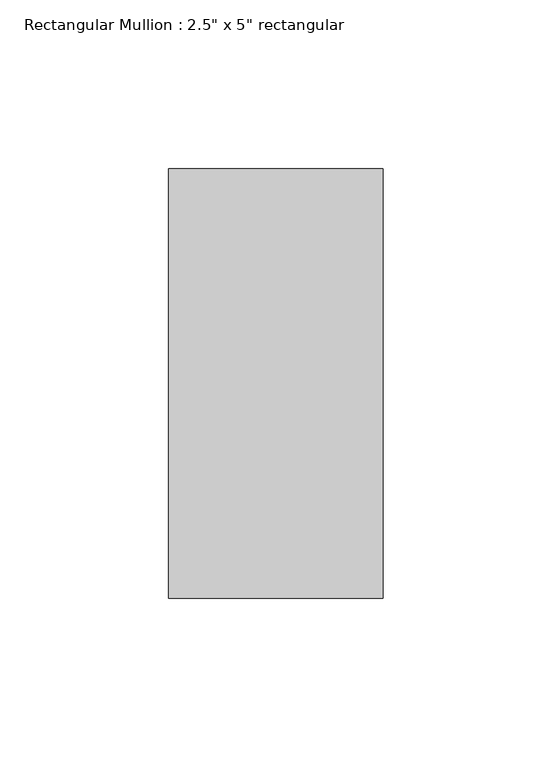
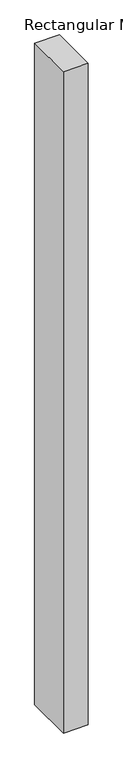
"""IFC4 building model written with IfcOpenShell, lengths in millimetres: member geometry."""

from ifc_helpers import new_model, si_unit, frame, origin, place, context, project, spatial, polyline, outline, extrude, source, transform, mapped, element, save


def member_49291f33(model_context):
    return source(origin(), model_context, "Body", "SweptSolid", [
        extrude(outline(polyline([(0.0, 63.5), (0.0, -63.5), (-63.5, -63.5), (-63.5, 63.5), (0.0, 63.5)])), frame((0.0, 0.0, -1789.0304763), z_axis=(0.0, 0.0, 1.0), x_axis=(1.0, 0.0, 0.0)), (0.0, 0.0, 1.0), 1789.0304763),
    ])


if __name__ == "__main__":
    model = new_model("IFC4")
    model_context = context("Model", 3, world=origin())
    ifc_project = project(units=[si_unit("LENGTHUNIT", "METRE", prefix="MILLI")], contexts=[model_context])
    site = spatial("IfcSite", under=ifc_project)
    building = spatial("IfcBuilding", under=site)
    placement = place(None, origin())
    member_shape = member_49291f33(model_context)
    element("IfcMember", 1, ObjectType="Rectangular Mullion : 2.5\" x 5\" rectangular", at=placement, inside=building, context=model_context, shape_type="MappedRepresentation", body=[
        mapped(member_shape, transform((0.0, 0.0, 0.0), x_axis=(1.0, 0.0, 0.0), y_axis=(0.0, 1.0, 0.0), z_axis=(0.0, 0.0, 1.0))),
    ])
    save(model, "model.ifc")

# Revit data of these elements
# Type "Rectangular Mullion : 2.5\" x 5\" rectangular"
#   built-in parameter 1007304 = 0.416667 (stored number, unit not read)
#   built-in parameter 1007301 = 0.104167 (stored number, unit not read)
#   built-in parameter 1007300 = 0.104167 (stored number, unit not read)
# Element 1 (IfcMember, "Rectangular Mullion : 2.5\" x 5\" rectangular")
#   Materials on its faces: "Aluminum"
# Materials
#   "Aluminum": class "Metal", colour RGB 247 247 247, transparency 0, Description = "Aluminum 6061", Cost = 0
